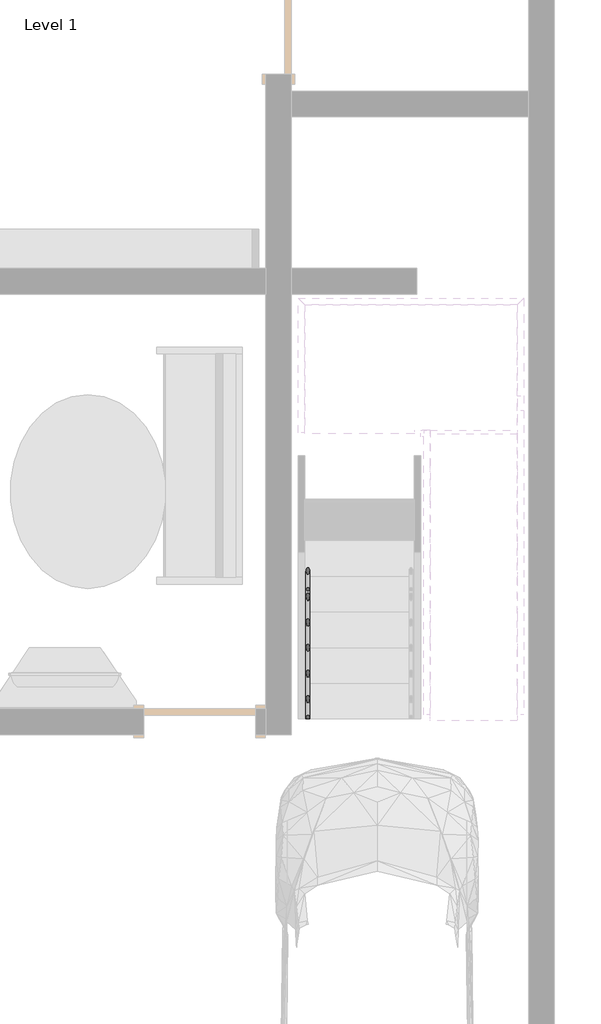
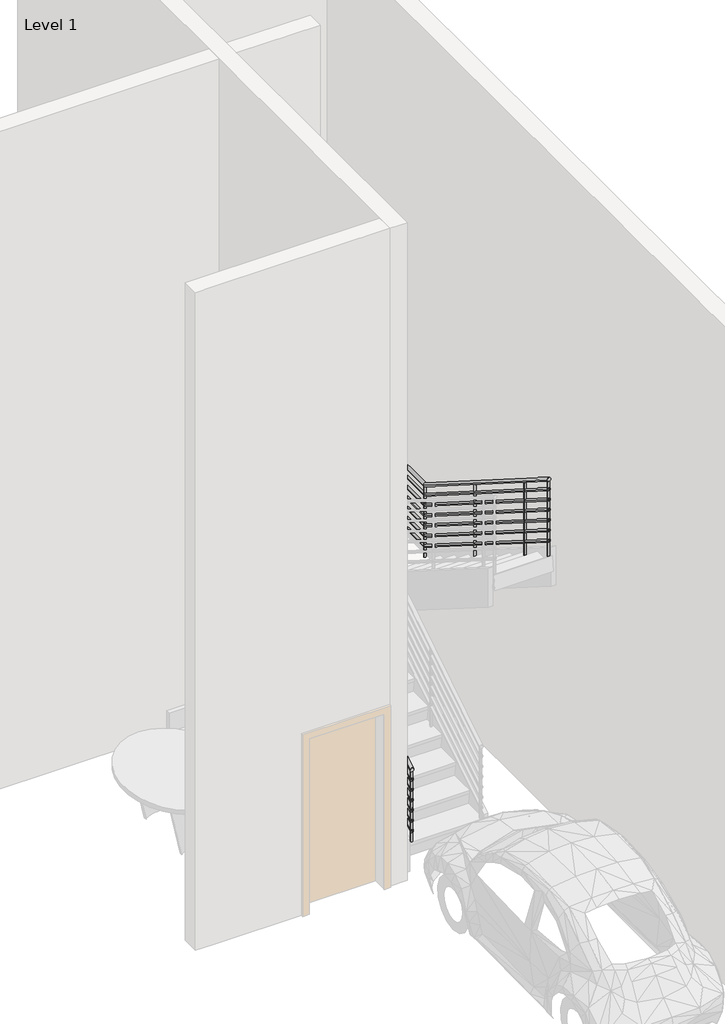
# One storey, part 3 of 4: 1 railing.
"""IFC4 building model written with IfcOpenShell, lengths in millimetres."""

from ifc_helpers import new_model, si_unit, point, frame, frame_2d, origin, place, context, project, spatial, circle_curve, ellipse_curve, trimmed, segment, composite_curve, outline, extrude, element, save
from ifc_brep_helpers import plane_surface, cylinder_surface, advanced_brep

model = new_model("IFC4")

# Units and contexts
model_context = context("Model", 3, world=origin())
ifc_project = project(units=[si_unit("LENGTHUNIT", "METRE", prefix="MILLI")], contexts=[model_context])

# Site, building, storey
site = spatial("IfcSite", under=ifc_project)
building = spatial("IfcBuilding", under=site)
storey = spatial("IfcBuildingStorey", under=building, Name="Level 1", Elevation=0.0)

# Railing
placement = place(None, origin())
element("IfcRailing", 1, ObjectType="900mm Pipe", at=placement, inside=storey, context=model_context, shape_type="SolidModel", body=[
    advanced_brep(
    [(-322.6389075, 5121.4805518, 1224.1622432), (-362.6389075, 5121.4805518, 1224.1622432), (-322.6389075, 7327.2740048, 2619.1304348), (-362.6389075, 7327.2740048, 2619.1304348), (-322.6389075, 8276.1063331, 2619.1304348), (-362.6389075, 8316.1063331, 2619.1304348), (1230.1786001, 8276.1063331, 2619.1304348), (1270.1786001, 8316.1063331, 2619.1304348), (1230.1786001, 7620.4870988, 2619.1304348), (1270.1786001, 7620.4870988, 2619.1304348), (1230.1786001, 5151.2805518, 4180.6839823), (1270.1786001, 5151.2805518, 4180.6839823)],
    [
        (0, 1, ellipse_curve(frame((-342.6389075, 5121.4805518, 1224.1622432), z_axis=(0.0, -1.0, 0.0), x_axis=(0.0, 0.0, -1.0)), 23.6638438, 20.0)),
        (1, 0, ellipse_curve(frame((-342.6389075, 5121.4805518, 1224.1622432), z_axis=(0.0, -1.0, 0.0), x_axis=(0.0, 0.0, -1.0)), 23.6638438, 20.0)),
        (0, 2),
        (2, 3, ellipse_curve(frame((-342.6389075, 7327.2740048, 2619.1304348), z_axis=(0.0, -0.9605132043335073, -0.27823440531497556), x_axis=(0.0, 0.2782344053149756, -0.9605132043335072)), 20.822202, 20.0)),
        (3, 1),
        (3, 2, ellipse_curve(frame((-342.6389075, 7327.2740048, 2619.1304348), z_axis=(0.0, -0.9605132043335073, -0.27823440531497556), x_axis=(0.0, 0.2782344053149756, -0.9605132043335072)), 20.822202, 20.0)),
        (2, 4),
        (4, 5, ellipse_curve(frame((-342.6389075, 8296.1063331, 2619.1304348), z_axis=(-0.707106781186549, -0.7071067811865458, 0.0), x_axis=(0.7071067811865457, -0.7071067811865495, 0.0)), 28.2842712, 20.0)),
        (5, 3),
        (5, 4, ellipse_curve(frame((-342.6389075, 8296.1063331, 2619.1304348), z_axis=(-0.707106781186549, -0.7071067811865458, 0.0), x_axis=(0.7071067811865457, -0.7071067811865495, 0.0)), 28.2842712, 20.0)),
        (4, 6),
        (6, 7, ellipse_curve(frame((1250.1786001, 8296.1063331, 2619.1304348), z_axis=(-0.7071067811865456, 0.7071067811865493, 0.0), x_axis=(-0.7071067811865495, -0.7071067811865456, 0.0)), 28.2842712, 20.0)),
        (7, 5),
        (7, 6, ellipse_curve(frame((1250.1786001, 8296.1063331, 2619.1304348), z_axis=(-0.7071067811865456, 0.7071067811865493, 0.0), x_axis=(-0.7071067811865495, -0.7071067811865456, 0.0)), 28.2842712, 20.0)),
        (6, 8),
        (8, 9, ellipse_curve(frame((1250.1786001, 7620.4870988, 2619.1304348), z_axis=(0.0, 0.9605132043335073, -0.2782344053149755), x_axis=(0.0, 0.2782344053149757, 0.9605132043335073)), 20.822202, 20.0)),
        (9, 7),
        (9, 8, ellipse_curve(frame((1250.1786001, 7620.4870988, 2619.1304348), z_axis=(0.0, 0.9605132043335073, -0.2782344053149755), x_axis=(0.0, 0.2782344053149757, 0.9605132043335073)), 20.822202, 20.0)),
        (10, 11, ellipse_curve(frame((1250.1786001, 5151.2805518, 4180.6839823), z_axis=(0.0, -1.0, 0.0), x_axis=(0.0, 0.0, -1.0)), 23.6638438, 20.0)),
        (11, 10, ellipse_curve(frame((1250.1786001, 5151.2805518, 4180.6839823), z_axis=(0.0, -1.0, 0.0), x_axis=(0.0, 0.0, -1.0)), 23.6638438, 20.0)),
        (8, 10),
        (11, 9),
    ],
    [
        plane_surface(frame((-342.6389075, 5121.4805518, 1247.826087), z_axis=(0.0, -1.0, 0.0), x_axis=(0.0, 0.0, 1.0))),
        cylinder_surface(frame((-342.6389075, 5132.1704646, 1230.9226623), z_axis=(0.0, -0.8451712313980438, -0.5344956404098301), x_axis=(-1.0, 0.0, 0.0)), 20.0),
        cylinder_surface(frame((-342.6389075, 7321.4805518, 2619.1304348), z_axis=(0.0, -1.0, 0.0), x_axis=(-1.0, 0.0, 0.0)), 20.0),
        cylinder_surface(frame((-342.6389075, 8296.1063331, 2619.1304348), z_axis=(-1.0, 0.0, 0.0), x_axis=(0.0, 1.0, 0.0)), 20.0),
        cylinder_surface(frame((1250.1786001, 8296.1063331, 2619.1304348), z_axis=(0.0, 1.0, 0.0), x_axis=(1.0, 0.0, 0.0)), 20.0),
        plane_surface(frame((1250.1786001, 5151.2805518, 4204.3478261), z_axis=(0.0, -1.0, 0.0), x_axis=(0.0, 0.0, -1.0))),
        cylinder_surface(frame((1250.1786001, 7615.590639, 2622.2270102), z_axis=(0.0, 0.8451712313980438, -0.53449564040983), x_axis=(1.0, 0.0, 0.0)), 20.0),
    ],
    [
        (0, [[1, 2]]),
        (1, [[-1, 3, 4, 5]]),
        (1, [[-2, -5, 6, -3]]),
        (2, [[-4, 7, 8, 9]]),
        (2, [[-6, -9, 10, -7]]),
        (3, [[-8, 11, 12, 13]]),
        (3, [[-10, -13, 14, -11]]),
        (4, [[-12, 15, 16, 17]]),
        (4, [[-14, -17, 18, -15]]),
        (5, [[19, 20]]),
        (6, [[-16, 21, -20, 22]]),
        (6, [[-18, -22, -19, -21]]),
    ],
),
    advanced_brep(
    [(-327.6389075, 5121.4805518, 1105.0782041), (-357.6389075, 5121.4805518, 1105.0782041), (-327.6389075, 7325.8256416, 2499.1304348), (-357.6389075, 7325.8256416, 2499.1304348), (-327.6389075, 8281.1063331, 2499.1304348), (-357.6389075, 8311.1063331, 2499.1304348), (1235.1786001, 8281.1063331, 2499.1304348), (1265.1786001, 8311.1063331, 2499.1304348), (1235.1786001, 7621.9354621, 2499.1304348), (1265.1786001, 7621.9354621, 2499.1304348), (1235.1786001, 5151.2805518, 4061.5999432), (1265.1786001, 5151.2805518, 4061.5999432)],
    [
        (0, 1, ellipse_curve(frame((-342.6389075, 5121.4805518, 1105.0782041), z_axis=(0.0, -1.0, 0.0), x_axis=(0.0, 0.0, -1.0)), 17.7478828, 15.0)),
        (1, 0, ellipse_curve(frame((-342.6389075, 5121.4805518, 1105.0782041), z_axis=(0.0, -1.0, 0.0), x_axis=(0.0, 0.0, -1.0)), 17.7478828, 15.0)),
        (0, 2),
        (2, 3, ellipse_curve(frame((-342.6389075, 7325.8256416, 2499.1304348), z_axis=(0.0, -0.9605132043335073, -0.27823440531497556), x_axis=(0.0, 0.2782344053149754, -0.9605132043335074)), 15.6166515, 15.0)),
        (3, 1),
        (3, 2, ellipse_curve(frame((-342.6389075, 7325.8256416, 2499.1304348), z_axis=(0.0, -0.9605132043335073, -0.27823440531497556), x_axis=(0.0, 0.2782344053149754, -0.9605132043335074)), 15.6166515, 15.0)),
        (2, 4),
        (4, 5, ellipse_curve(frame((-342.6389075, 8296.1063331, 2499.1304348), z_axis=(-0.707106781186549, -0.7071067811865458, 0.0), x_axis=(0.7071067811865457, -0.7071067811865495, 0.0)), 21.2132034, 15.0)),
        (5, 3),
        (5, 4, ellipse_curve(frame((-342.6389075, 8296.1063331, 2499.1304348), z_axis=(-0.707106781186549, -0.7071067811865458, 0.0), x_axis=(0.7071067811865457, -0.7071067811865495, 0.0)), 21.2132034, 15.0)),
        (4, 6),
        (6, 7, ellipse_curve(frame((1250.1786001, 8296.1063331, 2499.1304348), z_axis=(-0.7071067811865456, 0.7071067811865493, 0.0), x_axis=(-0.7071067811865495, -0.7071067811865456, 0.0)), 21.2132034, 15.0)),
        (7, 5),
        (7, 6, ellipse_curve(frame((1250.1786001, 8296.1063331, 2499.1304348), z_axis=(-0.7071067811865456, 0.7071067811865493, 0.0), x_axis=(-0.7071067811865495, -0.7071067811865456, 0.0)), 21.2132034, 15.0)),
        (6, 8),
        (8, 9, ellipse_curve(frame((1250.1786001, 7621.9354621, 2499.1304348), z_axis=(0.0, 0.9605132043335073, -0.27823440531497556), x_axis=(0.0, 0.27823440531497573, 0.9605132043335072)), 15.6166515, 15.0)),
        (9, 7),
        (9, 8, ellipse_curve(frame((1250.1786001, 7621.9354621, 2499.1304348), z_axis=(0.0, 0.9605132043335073, -0.27823440531497556), x_axis=(0.0, 0.27823440531497573, 0.9605132043335072)), 15.6166515, 15.0)),
        (10, 11, ellipse_curve(frame((1250.1786001, 5151.2805518, 4061.5999432), z_axis=(0.0, -1.0, 0.0), x_axis=(0.0, 0.0, -1.0)), 17.7478828, 15.0)),
        (11, 10, ellipse_curve(frame((1250.1786001, 5151.2805518, 4061.5999432), z_axis=(0.0, -1.0, 0.0), x_axis=(0.0, 0.0, -1.0)), 17.7478828, 15.0)),
        (8, 10),
        (11, 9),
    ],
    [
        plane_surface(frame((-342.6389075, 5121.4805518, 1122.826087), z_axis=(0.0, -1.0, 0.0), x_axis=(0.0, 0.0, 1.0))),
        cylinder_surface(frame((-342.6389075, 5129.4979864, 1110.1485185), z_axis=(0.0, -0.845171231398044, -0.53449564040983), x_axis=(-1.0, 0.0, 0.0)), 15.0),
        cylinder_surface(frame((-342.6389075, 7321.4805518, 2499.1304348), z_axis=(0.0, -1.0, 0.0), x_axis=(-1.0, 0.0, 0.0)), 15.0),
        cylinder_surface(frame((-342.6389075, 8296.1063331, 2499.1304348), z_axis=(-1.0, 0.0, 0.0), x_axis=(0.0, 1.0, 0.0)), 15.0),
        cylinder_surface(frame((1250.1786001, 8296.1063331, 2499.1304348), z_axis=(0.0, 1.0, 0.0), x_axis=(1.0, 0.0, 0.0)), 15.0),
        plane_surface(frame((1250.1786001, 5151.2805518, 4079.3478261), z_axis=(0.0, -1.0, 0.0), x_axis=(0.0, 0.0, -1.0))),
        cylinder_surface(frame((1250.1786001, 7618.2631172, 2501.4528663), z_axis=(0.0, 0.8451712313980438, -0.53449564040983), x_axis=(1.0, 0.0, 0.0)), 15.0),
    ],
    [
        (0, [[1, 2]]),
        (1, [[-1, 3, 4, 5]]),
        (1, [[-2, -5, 6, -3]]),
        (2, [[-4, 7, 8, 9]]),
        (2, [[-6, -9, 10, -7]]),
        (3, [[-8, 11, 12, 13]]),
        (3, [[-10, -13, 14, -11]]),
        (4, [[-12, 15, 16, 17]]),
        (4, [[-14, -17, 18, -15]]),
        (5, [[19, 20]]),
        (6, [[-16, 21, -20, 22]]),
        (6, [[-18, -22, -19, -21]]),
    ],
),
    advanced_brep(
    [(-327.6389075, 5121.4805518, 980.0782041), (-357.6389075, 5121.4805518, 980.0782041), (-327.6389075, 7325.8256416, 2374.1304348), (-357.6389075, 7325.8256416, 2374.1304348), (-327.6389075, 8281.1063331, 2374.1304348), (-357.6389075, 8311.1063331, 2374.1304348), (1235.1786001, 8281.1063331, 2374.1304348), (1265.1786001, 8311.1063331, 2374.1304348), (1235.1786001, 7621.9354621, 2374.1304348), (1265.1786001, 7621.9354621, 2374.1304348), (1235.1786001, 5151.2805518, 3936.5999432), (1265.1786001, 5151.2805518, 3936.5999432)],
    [
        (0, 1, ellipse_curve(frame((-342.6389075, 5121.4805518, 980.0782041), z_axis=(0.0, -1.0, 0.0), x_axis=(0.0, 0.0, -1.0)), 17.7478828, 15.0)),
        (1, 0, ellipse_curve(frame((-342.6389075, 5121.4805518, 980.0782041), z_axis=(0.0, -1.0, 0.0), x_axis=(0.0, 0.0, -1.0)), 17.7478828, 15.0)),
        (0, 2),
        (2, 3, ellipse_curve(frame((-342.6389075, 7325.8256416, 2374.1304348), z_axis=(0.0, -0.9605132043335073, -0.27823440531497556), x_axis=(0.0, 0.2782344053149756, -0.9605132043335072)), 15.6166515, 15.0)),
        (3, 1),
        (3, 2, ellipse_curve(frame((-342.6389075, 7325.8256416, 2374.1304348), z_axis=(0.0, -0.9605132043335073, -0.27823440531497556), x_axis=(0.0, 0.2782344053149756, -0.9605132043335072)), 15.6166515, 15.0)),
        (2, 4),
        (4, 5, ellipse_curve(frame((-342.6389075, 8296.1063331, 2374.1304348), z_axis=(-0.707106781186549, -0.7071067811865458, 0.0), x_axis=(0.7071067811865457, -0.7071067811865495, 0.0)), 21.2132034, 15.0)),
        (5, 3),
        (5, 4, ellipse_curve(frame((-342.6389075, 8296.1063331, 2374.1304348), z_axis=(-0.707106781186549, -0.7071067811865458, 0.0), x_axis=(0.7071067811865457, -0.7071067811865495, 0.0)), 21.2132034, 15.0)),
        (4, 6),
        (6, 7, ellipse_curve(frame((1250.1786001, 8296.1063331, 2374.1304348), z_axis=(-0.7071067811865456, 0.7071067811865493, 0.0), x_axis=(-0.7071067811865495, -0.7071067811865456, 0.0)), 21.2132034, 15.0)),
        (7, 5),
        (7, 6, ellipse_curve(frame((1250.1786001, 8296.1063331, 2374.1304348), z_axis=(-0.7071067811865456, 0.7071067811865493, 0.0), x_axis=(-0.7071067811865495, -0.7071067811865456, 0.0)), 21.2132034, 15.0)),
        (6, 8),
        (8, 9, ellipse_curve(frame((1250.1786001, 7621.9354621, 2374.1304348), z_axis=(0.0, 0.9605132043335073, -0.27823440531497545), x_axis=(0.0, 0.27823440531497573, 0.9605132043335072)), 15.6166515, 15.0)),
        (9, 7),
        (9, 8, ellipse_curve(frame((1250.1786001, 7621.9354621, 2374.1304348), z_axis=(0.0, 0.9605132043335073, -0.27823440531497545), x_axis=(0.0, 0.27823440531497573, 0.9605132043335072)), 15.6166515, 15.0)),
        (10, 11, ellipse_curve(frame((1250.1786001, 5151.2805518, 3936.5999432), z_axis=(0.0, -1.0, 0.0), x_axis=(0.0, 0.0, -1.0)), 17.7478828, 15.0)),
        (11, 10, ellipse_curve(frame((1250.1786001, 5151.2805518, 3936.5999432), z_axis=(0.0, -1.0, 0.0), x_axis=(0.0, 0.0, -1.0)), 17.7478828, 15.0)),
        (8, 10),
        (11, 9),
    ],
    [
        plane_surface(frame((-342.6389075, 5121.4805518, 997.826087), z_axis=(0.0, -1.0, 0.0), x_axis=(0.0, 0.0, 1.0))),
        cylinder_surface(frame((-342.6389075, 5129.4979864, 985.1485185), z_axis=(0.0, -0.8451712313980438, -0.5344956404098301), x_axis=(-1.0, 0.0, 0.0)), 15.0),
        cylinder_surface(frame((-342.6389075, 7321.4805518, 2374.1304348), z_axis=(0.0, -1.0, 0.0), x_axis=(-1.0, 0.0, 0.0)), 15.0),
        cylinder_surface(frame((-342.6389075, 8296.1063331, 2374.1304348), z_axis=(-1.0, 0.0, 0.0), x_axis=(0.0, 1.0, 0.0)), 15.0),
        cylinder_surface(frame((1250.1786001, 8296.1063331, 2374.1304348), z_axis=(0.0, 1.0, 0.0), x_axis=(1.0, 0.0, 0.0)), 15.0),
        plane_surface(frame((1250.1786001, 5151.2805518, 3954.3478261), z_axis=(0.0, -1.0, 0.0), x_axis=(0.0, 0.0, -1.0))),
        cylinder_surface(frame((1250.1786001, 7618.2631172, 2376.4528663), z_axis=(0.0, 0.845171231398044, -0.5344956404098299), x_axis=(1.0, 0.0, 0.0)), 15.0),
    ],
    [
        (0, [[1, 2]]),
        (1, [[-1, 3, 4, 5]]),
        (1, [[-2, -5, 6, -3]]),
        (2, [[-4, 7, 8, 9]]),
        (2, [[-6, -9, 10, -7]]),
        (3, [[-8, 11, 12, 13]]),
        (3, [[-10, -13, 14, -11]]),
        (4, [[-12, 15, 16, 17]]),
        (4, [[-14, -17, 18, -15]]),
        (5, [[19, 20]]),
        (6, [[-16, 21, -20, 22]]),
        (6, [[-18, -22, -19, -21]]),
    ],
),
    advanced_brep(
    [(-327.6389075, 5121.4805518, 855.0782041), (-357.6389075, 5121.4805518, 855.0782041), (-327.6389075, 7325.8256416, 2249.1304348), (-357.6389075, 7325.8256416, 2249.1304348), (-327.6389075, 8281.1063331, 2249.1304348), (-357.6389075, 8311.1063331, 2249.1304348), (1235.1786001, 8281.1063331, 2249.1304348), (1265.1786001, 8311.1063331, 2249.1304348), (1235.1786001, 7621.9354621, 2249.1304348), (1265.1786001, 7621.9354621, 2249.1304348), (1235.1786001, 5151.2805518, 3811.5999432), (1265.1786001, 5151.2805518, 3811.5999432)],
    [
        (0, 1, ellipse_curve(frame((-342.6389075, 5121.4805518, 855.0782041), z_axis=(0.0, -1.0, 0.0), x_axis=(0.0, 0.0, -1.0)), 17.7478828, 15.0)),
        (1, 0, ellipse_curve(frame((-342.6389075, 5121.4805518, 855.0782041), z_axis=(0.0, -1.0, 0.0), x_axis=(0.0, 0.0, -1.0)), 17.7478828, 15.0)),
        (0, 2),
        (2, 3, ellipse_curve(frame((-342.6389075, 7325.8256416, 2249.1304348), z_axis=(0.0, -0.9605132043335073, -0.27823440531497556), x_axis=(0.0, 0.2782344053149756, -0.9605132043335072)), 15.6166515, 15.0)),
        (3, 1),
        (3, 2, ellipse_curve(frame((-342.6389075, 7325.8256416, 2249.1304348), z_axis=(0.0, -0.9605132043335073, -0.27823440531497556), x_axis=(0.0, 0.2782344053149756, -0.9605132043335072)), 15.6166515, 15.0)),
        (2, 4),
        (4, 5, ellipse_curve(frame((-342.6389075, 8296.1063331, 2249.1304348), z_axis=(-0.707106781186549, -0.7071067811865458, 0.0), x_axis=(0.7071067811865457, -0.7071067811865495, 0.0)), 21.2132034, 15.0)),
        (5, 3),
        (5, 4, ellipse_curve(frame((-342.6389075, 8296.1063331, 2249.1304348), z_axis=(-0.707106781186549, -0.7071067811865458, 0.0), x_axis=(0.7071067811865457, -0.7071067811865495, 0.0)), 21.2132034, 15.0)),
        (4, 6),
        (6, 7, ellipse_curve(frame((1250.1786001, 8296.1063331, 2249.1304348), z_axis=(-0.7071067811865456, 0.7071067811865493, 0.0), x_axis=(-0.7071067811865495, -0.7071067811865456, 0.0)), 21.2132034, 15.0)),
        (7, 5),
        (7, 6, ellipse_curve(frame((1250.1786001, 8296.1063331, 2249.1304348), z_axis=(-0.7071067811865456, 0.7071067811865493, 0.0), x_axis=(-0.7071067811865495, -0.7071067811865456, 0.0)), 21.2132034, 15.0)),
        (6, 8),
        (8, 9, ellipse_curve(frame((1250.1786001, 7621.9354621, 2249.1304348), z_axis=(0.0, 0.9605132043335073, -0.27823440531497545), x_axis=(0.0, 0.27823440531497573, 0.9605132043335072)), 15.6166515, 15.0)),
        (9, 7),
        (9, 8, ellipse_curve(frame((1250.1786001, 7621.9354621, 2249.1304348), z_axis=(0.0, 0.9605132043335073, -0.27823440531497545), x_axis=(0.0, 0.27823440531497573, 0.9605132043335072)), 15.6166515, 15.0)),
        (10, 11, ellipse_curve(frame((1250.1786001, 5151.2805518, 3811.5999432), z_axis=(0.0, -1.0, 0.0), x_axis=(0.0, 0.0, -1.0)), 17.7478828, 15.0)),
        (11, 10, ellipse_curve(frame((1250.1786001, 5151.2805518, 3811.5999432), z_axis=(0.0, -1.0, 0.0), x_axis=(0.0, 0.0, -1.0)), 17.7478828, 15.0)),
        (8, 10),
        (11, 9),
    ],
    [
        plane_surface(frame((-342.6389075, 5121.4805518, 872.826087), z_axis=(0.0, -1.0, 0.0), x_axis=(0.0, 0.0, 1.0))),
        cylinder_surface(frame((-342.6389075, 5129.4979864, 860.1485185), z_axis=(0.0, -0.8451712313980438, -0.5344956404098301), x_axis=(-1.0, 0.0, 0.0)), 15.0),
        cylinder_surface(frame((-342.6389075, 7321.4805518, 2249.1304348), z_axis=(0.0, -1.0, 0.0), x_axis=(-1.0, 0.0, 0.0)), 15.0),
        cylinder_surface(frame((-342.6389075, 8296.1063331, 2249.1304348), z_axis=(-1.0, 0.0, 0.0), x_axis=(0.0, 1.0, 0.0)), 15.0),
        cylinder_surface(frame((1250.1786001, 8296.1063331, 2249.1304348), z_axis=(0.0, 1.0, 0.0), x_axis=(1.0, 0.0, 0.0)), 15.0),
        plane_surface(frame((1250.1786001, 5151.2805518, 3829.3478261), z_axis=(0.0, -1.0, 0.0), x_axis=(0.0, 0.0, -1.0))),
        cylinder_surface(frame((1250.1786001, 7618.2631172, 2251.4528663), z_axis=(0.0, 0.845171231398044, -0.5344956404098299), x_axis=(1.0, 0.0, 0.0)), 15.0),
    ],
    [
        (0, [[1, 2]]),
        (1, [[-1, 3, 4, 5]]),
        (1, [[-2, -5, 6, -3]]),
        (2, [[-4, 7, 8, 9]]),
        (2, [[-6, -9, 10, -7]]),
        (3, [[-8, 11, 12, 13]]),
        (3, [[-10, -13, 14, -11]]),
        (4, [[-12, 15, 16, 17]]),
        (4, [[-14, -17, 18, -15]]),
        (5, [[19, 20]]),
        (6, [[-16, 21, -20, 22]]),
        (6, [[-18, -22, -19, -21]]),
    ],
),
    advanced_brep(
    [(-327.6389075, 5121.4805518, 730.0782041), (-357.6389075, 5121.4805518, 730.0782041), (-327.6389075, 7325.8256416, 2124.1304348), (-357.6389075, 7325.8256416, 2124.1304348), (-327.6389075, 8281.1063331, 2124.1304348), (-357.6389075, 8311.1063331, 2124.1304348), (1235.1786001, 8281.1063331, 2124.1304348), (1265.1786001, 8311.1063331, 2124.1304348), (1235.1786001, 7621.9354621, 2124.1304348), (1265.1786001, 7621.9354621, 2124.1304348), (1235.1786001, 5151.2805518, 3686.5999432), (1265.1786001, 5151.2805518, 3686.5999432)],
    [
        (0, 1, ellipse_curve(frame((-342.6389075, 5121.4805518, 730.0782041), z_axis=(0.0, -1.0, 0.0), x_axis=(0.0, 0.0, -1.0)), 17.7478828, 15.0)),
        (1, 0, ellipse_curve(frame((-342.6389075, 5121.4805518, 730.0782041), z_axis=(0.0, -1.0, 0.0), x_axis=(0.0, 0.0, -1.0)), 17.7478828, 15.0)),
        (0, 2),
        (2, 3, ellipse_curve(frame((-342.6389075, 7325.8256416, 2124.1304348), z_axis=(0.0, -0.9605132043335073, -0.27823440531497556), x_axis=(0.0, 0.2782344053149756, -0.9605132043335072)), 15.6166515, 15.0)),
        (3, 1),
        (3, 2, ellipse_curve(frame((-342.6389075, 7325.8256416, 2124.1304348), z_axis=(0.0, -0.9605132043335073, -0.27823440531497556), x_axis=(0.0, 0.2782344053149756, -0.9605132043335072)), 15.6166515, 15.0)),
        (2, 4),
        (4, 5, ellipse_curve(frame((-342.6389075, 8296.1063331, 2124.1304348), z_axis=(-0.707106781186549, -0.7071067811865458, 0.0), x_axis=(0.7071067811865457, -0.7071067811865495, 0.0)), 21.2132034, 15.0)),
        (5, 3),
        (5, 4, ellipse_curve(frame((-342.6389075, 8296.1063331, 2124.1304348), z_axis=(-0.707106781186549, -0.7071067811865458, 0.0), x_axis=(0.7071067811865457, -0.7071067811865495, 0.0)), 21.2132034, 15.0)),
        (4, 6),
        (6, 7, ellipse_curve(frame((1250.1786001, 8296.1063331, 2124.1304348), z_axis=(-0.7071067811865456, 0.7071067811865493, 0.0), x_axis=(-0.7071067811865495, -0.7071067811865456, 0.0)), 21.2132034, 15.0)),
        (7, 5),
        (7, 6, ellipse_curve(frame((1250.1786001, 8296.1063331, 2124.1304348), z_axis=(-0.7071067811865456, 0.7071067811865493, 0.0), x_axis=(-0.7071067811865495, -0.7071067811865456, 0.0)), 21.2132034, 15.0)),
        (6, 8),
        (8, 9, ellipse_curve(frame((1250.1786001, 7621.9354621, 2124.1304348), z_axis=(0.0, 0.9605132043335073, -0.27823440531497545), x_axis=(0.0, 0.27823440531497573, 0.9605132043335072)), 15.6166515, 15.0)),
        (9, 7),
        (9, 8, ellipse_curve(frame((1250.1786001, 7621.9354621, 2124.1304348), z_axis=(0.0, 0.9605132043335073, -0.27823440531497545), x_axis=(0.0, 0.27823440531497573, 0.9605132043335072)), 15.6166515, 15.0)),
        (10, 11, ellipse_curve(frame((1250.1786001, 5151.2805518, 3686.5999432), z_axis=(0.0, -1.0, 0.0), x_axis=(0.0, 0.0, -1.0)), 17.7478828, 15.0)),
        (11, 10, ellipse_curve(frame((1250.1786001, 5151.2805518, 3686.5999432), z_axis=(0.0, -1.0, 0.0), x_axis=(0.0, 0.0, -1.0)), 17.7478828, 15.0)),
        (8, 10),
        (11, 9),
    ],
    [
        plane_surface(frame((-342.6389075, 5121.4805518, 747.826087), z_axis=(0.0, -1.0, 0.0), x_axis=(0.0, 0.0, 1.0))),
        cylinder_surface(frame((-342.6389075, 5129.4979864, 735.1485185), z_axis=(0.0, -0.8451712313980438, -0.5344956404098301), x_axis=(-1.0, 0.0, 0.0)), 15.0),
        cylinder_surface(frame((-342.6389075, 7321.4805518, 2124.1304348), z_axis=(0.0, -1.0, 0.0), x_axis=(-1.0, 0.0, 0.0)), 15.0),
        cylinder_surface(frame((-342.6389075, 8296.1063331, 2124.1304348), z_axis=(-1.0, 0.0, 0.0), x_axis=(0.0, 1.0, 0.0)), 15.0),
        cylinder_surface(frame((1250.1786001, 8296.1063331, 2124.1304348), z_axis=(0.0, 1.0, 0.0), x_axis=(1.0, 0.0, 0.0)), 15.0),
        plane_surface(frame((1250.1786001, 5151.2805518, 3704.3478261), z_axis=(0.0, -1.0, 0.0), x_axis=(0.0, 0.0, -1.0))),
        cylinder_surface(frame((1250.1786001, 7618.2631172, 2126.4528663), z_axis=(0.0, 0.845171231398044, -0.5344956404098299), x_axis=(1.0, 0.0, 0.0)), 15.0),
    ],
    [
        (0, [[1, 2]]),
        (1, [[-1, 3, 4, 5]]),
        (1, [[-2, -5, 6, -3]]),
        (2, [[-4, 7, 8, 9]]),
        (2, [[-6, -9, 10, -7]]),
        (3, [[-8, 11, 12, 13]]),
        (3, [[-10, -13, 14, -11]]),
        (4, [[-12, 15, 16, 17]]),
        (4, [[-14, -17, 18, -15]]),
        (5, [[19, 20]]),
        (6, [[-16, 21, -20, 22]]),
        (6, [[-18, -22, -19, -21]]),
    ],
),
    advanced_brep(
    [(-327.6389075, 5121.4805518, 605.0782041), (-357.6389075, 5121.4805518, 605.0782041), (-327.6389075, 7325.8256416, 1999.1304348), (-357.6389075, 7325.8256416, 1999.1304348), (-327.6389075, 8281.1063331, 1999.1304348), (-357.6389075, 8311.1063331, 1999.1304348), (1235.1786001, 8281.1063331, 1999.1304348), (1265.1786001, 8311.1063331, 1999.1304348), (1235.1786001, 7621.9354621, 1999.1304348), (1265.1786001, 7621.9354621, 1999.1304348), (1235.1786001, 5151.2805518, 3561.5999432), (1265.1786001, 5151.2805518, 3561.5999432)],
    [
        (0, 1, ellipse_curve(frame((-342.6389075, 5121.4805518, 605.0782041), z_axis=(0.0, -1.0, 0.0), x_axis=(0.0, 0.0, -1.0)), 17.7478828, 15.0)),
        (1, 0, ellipse_curve(frame((-342.6389075, 5121.4805518, 605.0782041), z_axis=(0.0, -1.0, 0.0), x_axis=(0.0, 0.0, -1.0)), 17.7478828, 15.0)),
        (0, 2),
        (2, 3, ellipse_curve(frame((-342.6389075, 7325.8256416, 1999.1304348), z_axis=(0.0, -0.9605132043335073, -0.27823440531497556), x_axis=(0.0, 0.2782344053149756, -0.9605132043335072)), 15.6166515, 15.0)),
        (3, 1),
        (3, 2, ellipse_curve(frame((-342.6389075, 7325.8256416, 1999.1304348), z_axis=(0.0, -0.9605132043335073, -0.27823440531497556), x_axis=(0.0, 0.2782344053149756, -0.9605132043335072)), 15.6166515, 15.0)),
        (2, 4),
        (4, 5, ellipse_curve(frame((-342.6389075, 8296.1063331, 1999.1304348), z_axis=(-0.707106781186549, -0.7071067811865458, 0.0), x_axis=(0.7071067811865457, -0.7071067811865495, 0.0)), 21.2132034, 15.0)),
        (5, 3),
        (5, 4, ellipse_curve(frame((-342.6389075, 8296.1063331, 1999.1304348), z_axis=(-0.707106781186549, -0.7071067811865458, 0.0), x_axis=(0.7071067811865457, -0.7071067811865495, 0.0)), 21.2132034, 15.0)),
        (4, 6),
        (6, 7, ellipse_curve(frame((1250.1786001, 8296.1063331, 1999.1304348), z_axis=(-0.7071067811865456, 0.7071067811865493, 0.0), x_axis=(-0.7071067811865495, -0.7071067811865456, 0.0)), 21.2132034, 15.0)),
        (7, 5),
        (7, 6, ellipse_curve(frame((1250.1786001, 8296.1063331, 1999.1304348), z_axis=(-0.7071067811865456, 0.7071067811865493, 0.0), x_axis=(-0.7071067811865495, -0.7071067811865456, 0.0)), 21.2132034, 15.0)),
        (6, 8),
        (8, 9, ellipse_curve(frame((1250.1786001, 7621.9354621, 1999.1304348), z_axis=(0.0, 0.9605132043335073, -0.2782344053149755), x_axis=(0.0, 0.2782344053149757, 0.9605132043335073)), 15.6166515, 15.0)),
        (9, 7),
        (9, 8, ellipse_curve(frame((1250.1786001, 7621.9354621, 1999.1304348), z_axis=(0.0, 0.9605132043335073, -0.2782344053149755), x_axis=(0.0, 0.2782344053149757, 0.9605132043335073)), 15.6166515, 15.0)),
        (10, 11, ellipse_curve(frame((1250.1786001, 5151.2805518, 3561.5999432), z_axis=(0.0, -1.0, 0.0), x_axis=(0.0, 0.0, -1.0)), 17.7478828, 15.0)),
        (11, 10, ellipse_curve(frame((1250.1786001, 5151.2805518, 3561.5999432), z_axis=(0.0, -1.0, 0.0), x_axis=(0.0, 0.0, -1.0)), 17.7478828, 15.0)),
        (8, 10),
        (11, 9),
    ],
    [
        plane_surface(frame((-342.6389075, 5121.4805518, 622.826087), z_axis=(0.0, -1.0, 0.0), x_axis=(0.0, 0.0, 1.0))),
        cylinder_surface(frame((-342.6389075, 5129.4979864, 610.1485185), z_axis=(0.0, -0.8451712313980438, -0.5344956404098301), x_axis=(-1.0, 0.0, 0.0)), 15.0),
        cylinder_surface(frame((-342.6389075, 7321.4805518, 1999.1304348), z_axis=(0.0, -1.0, 0.0), x_axis=(-1.0, 0.0, 0.0)), 15.0),
        cylinder_surface(frame((-342.6389075, 8296.1063331, 1999.1304348), z_axis=(-1.0, 0.0, 0.0), x_axis=(0.0, 1.0, 0.0)), 15.0),
        cylinder_surface(frame((1250.1786001, 8296.1063331, 1999.1304348), z_axis=(0.0, 1.0, 0.0), x_axis=(1.0, 0.0, 0.0)), 15.0),
        plane_surface(frame((1250.1786001, 5151.2805518, 3579.3478261), z_axis=(0.0, -1.0, 0.0), x_axis=(0.0, 0.0, -1.0))),
        cylinder_surface(frame((1250.1786001, 7618.2631172, 2001.4528663), z_axis=(0.0, 0.8451712313980438, -0.53449564040983), x_axis=(1.0, 0.0, 0.0)), 15.0),
    ],
    [
        (0, [[1, 2]]),
        (1, [[-1, 3, 4, 5]]),
        (1, [[-2, -5, 6, -3]]),
        (2, [[-4, 7, 8, 9]]),
        (2, [[-6, -9, 10, -7]]),
        (3, [[-8, 11, 12, 13]]),
        (3, [[-10, -13, 14, -11]]),
        (4, [[-12, 15, 16, 17]]),
        (4, [[-14, -17, 18, -15]]),
        (5, [[19, 20]]),
        (6, [[-16, 21, -20, 22]]),
        (6, [[-18, -22, -19, -21]]),
    ],
),
    advanced_brep(
    [(-327.6389075, 5121.4805518, 480.0782041), (-357.6389075, 5121.4805518, 480.0782041), (-327.6389075, 7325.8256416, 1874.1304348), (-357.6389075, 7325.8256416, 1874.1304348), (-327.6389075, 8281.1063331, 1874.1304348), (-357.6389075, 8311.1063331, 1874.1304348), (1235.1786001, 8281.1063331, 1874.1304348), (1265.1786001, 8311.1063331, 1874.1304348), (1235.1786001, 7621.9354621, 1874.1304348), (1265.1786001, 7621.9354621, 1874.1304348), (1235.1786001, 5151.2805518, 3436.5999432), (1265.1786001, 5151.2805518, 3436.5999432)],
    [
        (0, 1, ellipse_curve(frame((-342.6389075, 5121.4805518, 480.0782041), z_axis=(0.0, -1.0, 0.0), x_axis=(0.0, 0.0, -1.0)), 17.7478828, 15.0)),
        (1, 0, ellipse_curve(frame((-342.6389075, 5121.4805518, 480.0782041), z_axis=(0.0, -1.0, 0.0), x_axis=(0.0, 0.0, -1.0)), 17.7478828, 15.0)),
        (0, 2),
        (2, 3, ellipse_curve(frame((-342.6389075, 7325.8256416, 1874.1304348), z_axis=(0.0, -0.9605132043335073, -0.27823440531497556), x_axis=(0.0, 0.2782344053149756, -0.9605132043335072)), 15.6166515, 15.0)),
        (3, 1),
        (3, 2, ellipse_curve(frame((-342.6389075, 7325.8256416, 1874.1304348), z_axis=(0.0, -0.9605132043335073, -0.27823440531497556), x_axis=(0.0, 0.2782344053149756, -0.9605132043335072)), 15.6166515, 15.0)),
        (2, 4),
        (4, 5, ellipse_curve(frame((-342.6389075, 8296.1063331, 1874.1304348), z_axis=(-0.707106781186549, -0.7071067811865458, 0.0), x_axis=(0.7071067811865457, -0.7071067811865495, 0.0)), 21.2132034, 15.0)),
        (5, 3),
        (5, 4, ellipse_curve(frame((-342.6389075, 8296.1063331, 1874.1304348), z_axis=(-0.707106781186549, -0.7071067811865458, 0.0), x_axis=(0.7071067811865457, -0.7071067811865495, 0.0)), 21.2132034, 15.0)),
        (4, 6),
        (6, 7, ellipse_curve(frame((1250.1786001, 8296.1063331, 1874.1304348), z_axis=(-0.7071067811865456, 0.7071067811865493, 0.0), x_axis=(-0.7071067811865495, -0.7071067811865456, 0.0)), 21.2132034, 15.0)),
        (7, 5),
        (7, 6, ellipse_curve(frame((1250.1786001, 8296.1063331, 1874.1304348), z_axis=(-0.7071067811865456, 0.7071067811865493, 0.0), x_axis=(-0.7071067811865495, -0.7071067811865456, 0.0)), 21.2132034, 15.0)),
        (6, 8),
        (8, 9, ellipse_curve(frame((1250.1786001, 7621.9354621, 1874.1304348), z_axis=(0.0, 0.9605132043335073, -0.27823440531497545), x_axis=(0.0, 0.27823440531497573, 0.9605132043335072)), 15.6166515, 15.0)),
        (9, 7),
        (9, 8, ellipse_curve(frame((1250.1786001, 7621.9354621, 1874.1304348), z_axis=(0.0, 0.9605132043335073, -0.27823440531497545), x_axis=(0.0, 0.27823440531497573, 0.9605132043335072)), 15.6166515, 15.0)),
        (10, 11, ellipse_curve(frame((1250.1786001, 5151.2805518, 3436.5999432), z_axis=(0.0, -1.0, 0.0), x_axis=(0.0, 0.0, -1.0)), 17.7478828, 15.0)),
        (11, 10, ellipse_curve(frame((1250.1786001, 5151.2805518, 3436.5999432), z_axis=(0.0, -1.0, 0.0), x_axis=(0.0, 0.0, -1.0)), 17.7478828, 15.0)),
        (8, 10),
        (11, 9),
    ],
    [
        plane_surface(frame((-342.6389075, 5121.4805518, 497.826087), z_axis=(0.0, -1.0, 0.0), x_axis=(0.0, 0.0, 1.0))),
        cylinder_surface(frame((-342.6389075, 5129.4979864, 485.1485185), z_axis=(0.0, -0.8451712313980438, -0.5344956404098301), x_axis=(-1.0, 0.0, 0.0)), 15.0),
        cylinder_surface(frame((-342.6389075, 7321.4805518, 1874.1304348), z_axis=(0.0, -1.0, 0.0), x_axis=(-1.0, 0.0, 0.0)), 15.0),
        cylinder_surface(frame((-342.6389075, 8296.1063331, 1874.1304348), z_axis=(-1.0, 0.0, 0.0), x_axis=(0.0, 1.0, 0.0)), 15.0),
        cylinder_surface(frame((1250.1786001, 8296.1063331, 1874.1304348), z_axis=(0.0, 1.0, 0.0), x_axis=(1.0, 0.0, 0.0)), 15.0),
        plane_surface(frame((1250.1786001, 5151.2805518, 3454.3478261), z_axis=(0.0, -1.0, 0.0), x_axis=(0.0, 0.0, -1.0))),
        cylinder_surface(frame((1250.1786001, 7618.2631172, 1876.4528663), z_axis=(0.0, 0.845171231398044, -0.5344956404098299), x_axis=(1.0, 0.0, 0.0)), 15.0),
    ],
    [
        (0, [[1, 2]]),
        (1, [[-1, 3, 4, 5]]),
        (1, [[-2, -5, 6, -3]]),
        (2, [[-4, 7, 8, 9]]),
        (2, [[-6, -9, 10, -7]]),
        (3, [[-8, 11, 12, 13]]),
        (3, [[-10, -13, 14, -11]]),
        (4, [[-12, 15, 16, 17]]),
        (4, [[-14, -17, 18, -15]]),
        (5, [[19, 20]]),
        (6, [[-16, 21, -20, 22]]),
        (6, [[-18, -22, -19, -21]]),
    ],
),
    advanced_brep(
    [(1262.6786001, 5626.2805518, 3856.6248816), (1237.6786001, 5626.2805518, 3856.6248816), (1237.6786001, 5626.2805518, 2956.5217391), (1262.6786001, 5626.2805518, 2956.5217391)],
    [
        (0, 1, ellipse_curve(frame((1250.1786001, 5626.2805518, 3856.6248816), z_axis=(0.0, -0.5344956404098302, -0.8451712313980437), x_axis=(0.0, -0.8451712313980437, 0.53449564040983)), 14.7899024, 12.5)),
        (1, 2),
        (2, 3, circle_curve(frame((1250.1786001, 5626.2805518, 2956.5217391), z_axis=(0.0, 0.0, 1.0), x_axis=(-1.0, 0.0, 0.0)), 12.5)),
        (3, 0),
        (3, 2, circle_curve(frame((1250.1786001, 5626.2805518, 2956.5217391), z_axis=(0.0, 0.0, 1.0), x_axis=(-1.0, 0.0, 0.0)), 12.5)),
        (1, 0, ellipse_curve(frame((1250.1786001, 5626.2805518, 3856.6248816), z_axis=(0.0, -0.5344956404098302, -0.8451712313980437), x_axis=(0.0, -0.8451712313980437, 0.53449564040983)), 14.7899024, 12.5)),
    ],
    [
        cylinder_surface(frame((1250.1786001, 5626.2805518, 2856.5217391), z_axis=(0.0, 0.0, 1.0), x_axis=(-1.0, 0.0, 0.0)), 12.5),
        plane_surface(frame((1225.1786001, 5601.2805518, 3872.4351583), z_axis=(0.0, 0.5344956404098302, 0.8451712313980437), x_axis=(1.0, 0.0, 0.0))),
        plane_surface(frame((1225.1786001, 5651.2805518, 2956.5217391), z_axis=(0.0, 0.0, -1.0), x_axis=(1.0, 0.0, 0.0))),
    ],
    [
        (0, [[1, 2, 3, 4]]),
        (0, [[5, -2, 6, -4]]),
        (1, [[-6, -1]]),
        (2, [[-5, -3]]),
    ],
),
    advanced_brep(
    [(1262.6786001, 6626.2805518, 3224.2138144), (1237.6786001, 6626.2805518, 3224.2138144), (1237.6786001, 6626.2805518, 2260.8695652), (1262.6786001, 6626.2805518, 2260.8695652)],
    [
        (0, 1, ellipse_curve(frame((1250.1786001, 6626.2805518, 3224.2138144), z_axis=(0.0, -0.5344956404098302, -0.8451712313980437), x_axis=(0.0, -0.8451712313980437, 0.53449564040983)), 14.7899024, 12.5)),
        (1, 2),
        (2, 3, circle_curve(frame((1250.1786001, 6626.2805518, 2260.8695652), z_axis=(0.0, 0.0, 1.0), x_axis=(-1.0, 0.0, 0.0)), 12.5)),
        (3, 0),
        (3, 2, circle_curve(frame((1250.1786001, 6626.2805518, 2260.8695652), z_axis=(0.0, 0.0, 1.0), x_axis=(-1.0, 0.0, 0.0)), 12.5)),
        (1, 0, ellipse_curve(frame((1250.1786001, 6626.2805518, 3224.2138144), z_axis=(0.0, -0.5344956404098302, -0.8451712313980437), x_axis=(0.0, -0.8451712313980437, 0.53449564040983)), 14.7899024, 12.5)),
    ],
    [
        cylinder_surface(frame((1250.1786001, 6626.2805518, 2160.8695652), z_axis=(0.0, 0.0, 1.0), x_axis=(-1.0, 0.0, 0.0)), 12.5),
        plane_surface(frame((1225.1786001, 6601.2805518, 3240.0240911), z_axis=(0.0, 0.5344956404098302, 0.8451712313980437), x_axis=(1.0, 0.0, 0.0))),
        plane_surface(frame((1225.1786001, 6651.2805518, 2260.8695652), z_axis=(0.0, 0.0, -1.0), x_axis=(1.0, 0.0, 0.0))),
    ],
    [
        (0, [[1, 2, 3, 4]]),
        (0, [[5, -2, 6, -4]]),
        (1, [[-6, -1]]),
        (2, [[-5, -3]]),
    ],
),
    extrude(outline(composite_curve([segment(trimmed(circle_curve(frame_2d((657.3610925, 8296.1063331)), 12.5), [point((657.3610925, 8283.6063331))], [point((657.3610925, 8308.6063331))], False, "CARTESIAN"), True, "CONTINUOUS"), segment(trimmed(circle_curve(frame_2d((657.3610925, 8296.1063331)), 12.5), [point((657.3610925, 8308.6063331))], [point((657.3610925, 8283.6063331))], False, "CARTESIAN"), True, "CONTINUOUS")], self_intersect=False)), frame((0.0, 0.0, 1739.1304348), z_axis=(0.0, 0.0, 1.0), x_axis=(1.0, 0.0, 0.0)), (0.0, 0.0, 1.0), 860.0),
    advanced_brep(
    [(-355.1389075, 7121.4805518, 2465.3205338), (-330.1389075, 7121.4805518, 2465.3205338), (-330.1389075, 7121.4805518, 1565.2173913), (-355.1389075, 7121.4805518, 1565.2173913)],
    [
        (0, 1, ellipse_curve(frame((-342.6389075, 7121.4805518, 2465.3205338), z_axis=(0.0, 0.5344956404098302, -0.8451712313980437), x_axis=(0.0, 0.8451712313980437, 0.53449564040983)), 14.7899024, 12.5)),
        (1, 2),
        (2, 3, circle_curve(frame((-342.6389075, 7121.4805518, 1565.2173913), z_axis=(0.0, 0.0, 1.0), x_axis=(1.0, 0.0, 0.0)), 12.5)),
        (3, 0),
        (3, 2, circle_curve(frame((-342.6389075, 7121.4805518, 1565.2173913), z_axis=(0.0, 0.0, 1.0), x_axis=(1.0, 0.0, 0.0)), 12.5)),
        (1, 0, ellipse_curve(frame((-342.6389075, 7121.4805518, 2465.3205338), z_axis=(0.0, 0.5344956404098302, -0.8451712313980437), x_axis=(0.0, 0.8451712313980437, 0.53449564040983)), 14.7899024, 12.5)),
    ],
    [
        cylinder_surface(frame((-342.6389075, 7121.4805518, 1465.2173913), z_axis=(0.0, 0.0, 1.0), x_axis=(1.0, 0.0, 0.0)), 12.5),
        plane_surface(frame((-317.6389075, 7146.4805518, 2481.1308104), z_axis=(0.0, -0.5344956404098302, 0.8451712313980437), x_axis=(-1.0, 0.0, 0.0))),
        plane_surface(frame((-317.6389075, 7096.4805518, 1565.2173913), z_axis=(0.0, 0.0, -1.0), x_axis=(-1.0, 0.0, 0.0))),
    ],
    [
        (0, [[1, 2, 3, 4]]),
        (0, [[5, -2, 6, -4]]),
        (1, [[-6, -1]]),
        (2, [[-5, -3]]),
    ],
),
    advanced_brep(
    [(-355.1389075, 6121.4805518, 1832.9094666), (-330.1389075, 6121.4805518, 1832.9094666), (-330.1389075, 6121.4805518, 869.5652174), (-355.1389075, 6121.4805518, 869.5652174)],
    [
        (0, 1, ellipse_curve(frame((-342.6389075, 6121.4805518, 1832.9094666), z_axis=(0.0, 0.5344956404098302, -0.8451712313980437), x_axis=(0.0, 0.8451712313980437, 0.53449564040983)), 14.7899024, 12.5)),
        (1, 2),
        (2, 3, circle_curve(frame((-342.6389075, 6121.4805518, 869.5652174), z_axis=(0.0, 0.0, 1.0), x_axis=(1.0, 0.0, 0.0)), 12.5)),
        (3, 0),
        (3, 2, circle_curve(frame((-342.6389075, 6121.4805518, 869.5652174), z_axis=(0.0, 0.0, 1.0), x_axis=(1.0, 0.0, 0.0)), 12.5)),
        (1, 0, ellipse_curve(frame((-342.6389075, 6121.4805518, 1832.9094666), z_axis=(0.0, 0.5344956404098302, -0.8451712313980437), x_axis=(0.0, 0.8451712313980437, 0.53449564040983)), 14.7899024, 12.5)),
    ],
    [
        cylinder_surface(frame((-342.6389075, 6121.4805518, 769.5652174), z_axis=(0.0, 0.0, 1.0), x_axis=(1.0, 0.0, 0.0)), 12.5),
        plane_surface(frame((-317.6389075, 6146.4805518, 1848.7197432), z_axis=(0.0, -0.5344956404098302, 0.8451712313980437), x_axis=(-1.0, 0.0, 0.0))),
        plane_surface(frame((-317.6389075, 6096.4805518, 869.5652174), z_axis=(0.0, 0.0, -1.0), x_axis=(-1.0, 0.0, 0.0))),
    ],
    [
        (0, [[1, 2, 3, 4]]),
        (0, [[5, -2, 6, -4]]),
        (1, [[-6, -1]]),
        (2, [[-5, -3]]),
    ],
),
    extrude(outline(composite_curve([segment(trimmed(circle_curve(frame_2d((1250.1786001, 7626.2805518)), 12.5), [point((1237.6786001, 7626.2805518))], [point((1262.6786001, 7626.2805518))], False, "CARTESIAN"), True, "CONTINUOUS"), segment(trimmed(circle_curve(frame_2d((1250.1786001, 7626.2805518)), 12.5), [point((1262.6786001, 7626.2805518))], [point((1237.6786001, 7626.2805518))], False, "CARTESIAN"), True, "CONTINUOUS")], self_intersect=False)), frame((0.0, 0.0, 1739.1304348), z_axis=(0.0, 0.0, 1.0), x_axis=(1.0, 0.0, 0.0)), (0.0, 0.0, 1.0), 860.0),
    extrude(outline(composite_curve([segment(trimmed(circle_curve(frame_2d((1250.1786001, 8296.1063331)), 12.5), [point((1250.1786001, 8283.6063331))], [point((1250.1786001, 8308.6063331))], False, "CARTESIAN"), True, "CONTINUOUS"), segment(trimmed(circle_curve(frame_2d((1250.1786001, 8296.1063331)), 12.5), [point((1250.1786001, 8308.6063331))], [point((1250.1786001, 8283.6063331))], False, "CARTESIAN"), True, "CONTINUOUS")], self_intersect=False)), frame((0.0, 0.0, 1739.1304348), z_axis=(0.0, 0.0, 1.0), x_axis=(1.0, 0.0, 0.0)), (0.0, 0.0, 1.0), 860.0),
    extrude(outline(composite_curve([segment(trimmed(circle_curve(frame_2d((-342.6389075, 8296.1063331)), 12.5), [point((-330.1389075, 8296.1063331))], [point((-355.1389075, 8296.1063331))], False, "CARTESIAN"), True, "CONTINUOUS"), segment(trimmed(circle_curve(frame_2d((-342.6389075, 8296.1063331)), 12.5), [point((-355.1389075, 8296.1063331))], [point((-330.1389075, 8296.1063331))], False, "CARTESIAN"), True, "CONTINUOUS")], self_intersect=False)), frame((0.0, 0.0, 1739.1304348), z_axis=(0.0, 0.0, 1.0), x_axis=(1.0, 0.0, 0.0)), (0.0, 0.0, 1.0), 860.0),
    extrude(outline(composite_curve([segment(trimmed(circle_curve(frame_2d((-342.6389075, 7321.4805518)), 12.5), [point((-330.1389075, 7321.4805518))], [point((-355.1389075, 7321.4805518))], False, "CARTESIAN"), True, "CONTINUOUS"), segment(trimmed(circle_curve(frame_2d((-342.6389075, 7321.4805518)), 12.5), [point((-355.1389075, 7321.4805518))], [point((-330.1389075, 7321.4805518))], False, "CARTESIAN"), True, "CONTINUOUS")], self_intersect=False)), frame((0.0, 0.0, 1739.1304348), z_axis=(0.0, 0.0, 1.0), x_axis=(1.0, 0.0, 0.0)), (0.0, 0.0, 1.0), 860.0),
    advanced_brep(
    [(1262.6786001, 5163.7805518, 4149.1150002), (1237.6786001, 5163.7805518, 4149.1150002), (1237.6786001, 5163.7805518, 3130.4347826), (1262.6786001, 5163.7805518, 3130.4347826)],
    [
        (0, 1, ellipse_curve(frame((1250.1786001, 5163.7805518, 4149.1150002), z_axis=(0.0, -0.5344956404098302, -0.8451712313980437), x_axis=(0.0, -0.8451712313980437, 0.53449564040983)), 14.7899024, 12.5)),
        (1, 2),
        (2, 3, circle_curve(frame((1250.1786001, 5163.7805518, 3130.4347826), z_axis=(0.0, 0.0, 1.0), x_axis=(-1.0, 0.0, 0.0)), 12.5)),
        (3, 0),
        (3, 2, circle_curve(frame((1250.1786001, 5163.7805518, 3130.4347826), z_axis=(0.0, 0.0, 1.0), x_axis=(-1.0, 0.0, 0.0)), 12.5)),
        (1, 0, ellipse_curve(frame((1250.1786001, 5163.7805518, 4149.1150002), z_axis=(0.0, -0.5344956404098302, -0.8451712313980437), x_axis=(0.0, -0.8451712313980437, 0.53449564040983)), 14.7899024, 12.5)),
    ],
    [
        cylinder_surface(frame((1250.1786001, 5163.7805518, 3030.4347826), z_axis=(0.0, 0.0, 1.0), x_axis=(-1.0, 0.0, 0.0)), 12.5),
        plane_surface(frame((1225.1786001, 5138.7805518, 4164.9252768), z_axis=(0.0, 0.5344956404098302, 0.8451712313980437), x_axis=(1.0, 0.0, 0.0))),
        plane_surface(frame((1225.1786001, 5188.7805518, 3130.4347826), z_axis=(0.0, 0.0, -1.0), x_axis=(1.0, 0.0, 0.0))),
    ],
    [
        (0, [[1, 2, 3, 4]]),
        (0, [[5, -2, 6, -4]]),
        (1, [[-6, -1]]),
        (2, [[-5, -3]]),
    ],
),
    advanced_brep(
    [(-355.1389075, 5133.9805518, 1208.4035377), (-330.1389075, 5133.9805518, 1208.4035377), (-330.1389075, 5133.9805518, 347.826087), (-355.1389075, 5133.9805518, 347.826087)],
    [
        (0, 1, ellipse_curve(frame((-342.6389075, 5133.9805518, 1208.4035377), z_axis=(0.0, 0.5344956404098286, -0.8451712313980447), x_axis=(0.0, 0.8451712313980447, 0.5344956404098286)), 14.7899024, 12.5)),
        (1, 2),
        (2, 3, circle_curve(frame((-342.6389075, 5133.9805518, 347.826087), z_axis=(0.0, 0.0, 1.0), x_axis=(1.0, 0.0, 0.0)), 12.5)),
        (3, 0),
        (3, 2, circle_curve(frame((-342.6389075, 5133.9805518, 347.826087), z_axis=(0.0, 0.0, 1.0), x_axis=(1.0, 0.0, 0.0)), 12.5)),
        (1, 0, ellipse_curve(frame((-342.6389075, 5133.9805518, 1208.4035377), z_axis=(0.0, 0.5344956404098286, -0.8451712313980447), x_axis=(0.0, 0.8451712313980447, 0.5344956404098286)), 14.7899024, 12.5)),
    ],
    [
        cylinder_surface(frame((-342.6389075, 5133.9805518, 247.826087), z_axis=(0.0, 0.0, 1.0), x_axis=(1.0, 0.0, 0.0)), 12.5),
        plane_surface(frame((-317.6389075, 5158.9805518, 1224.2138144), z_axis=(0.0, -0.5344956404098286, 0.8451712313980447), x_axis=(-1.0, 0.0, 0.0))),
        plane_surface(frame((-317.6389075, 5108.9805518, 347.826087), z_axis=(0.0, 0.0, -1.0), x_axis=(-1.0, 0.0, 0.0))),
    ],
    [
        (0, [[1, 2, 3, 4]]),
        (0, [[5, -2, 6, -4]]),
        (1, [[-6, -1]]),
        (2, [[-5, -3]]),
    ],
),
])

save(model, "model.ifc")

# Revit data of these elements
# Type "900mm Pipe"
#   built-in parameter 1008612 = 0.019685 (stored number, unit not read)
#   built-in parameter 1008611 = 0.0984252 (stored number, unit not read)
#   built-in parameter 1008609 = 6.56168 (stored number, unit not read)
#   built-in parameter 1008604 = 0.19685 (stored number, unit not read)
#   built-in parameter 1008603 = 0.164042 (stored number, unit not read)
#   Railing Height = 900 mm
#   built-in parameter 1008630 = 2
#   built-in parameter 1008610 = 2
#   built-in parameter 1008605 = 1
#   built-in parameter 1008618 = M_Baluster - Round : 25mm
# Element 1 (IfcRailing, "900mm Pipe")
#   Phase Created = New Construction
